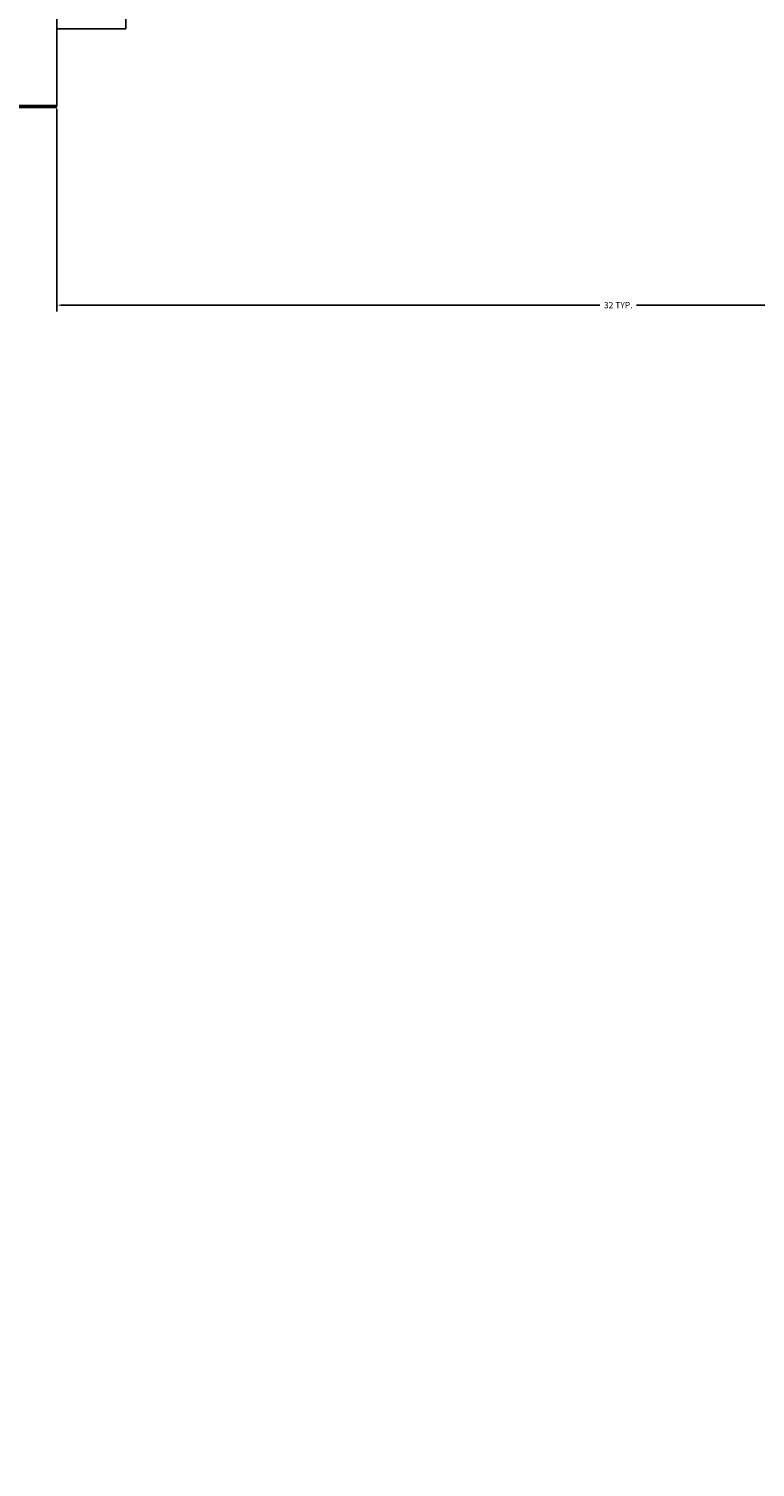
# Model space of a CAD drawing. Units: inches. Extents: x 963 to 2075, y 289 to 2657.
# Tile 92 of 98: x 1767 to 1788, y 2283 to 2325. Entities that reach past the tile are written whole.
import ezdxf

# ---------------------------------------------------------------- set-up
doc = ezdxf.new("R2010")
doc.units = ezdxf.units.IN
for name, color, linetype, lineweight in [('A-ANNO-DIMS', 2, 'Continuous', 18), ('A-DOOR', 4, 'Continuous', 25), ('A-WALL', 7, 'Continuous', 50), ('A-WALL-PATT', 8, 'Continuous', 13)]:
    doc.layers.add(name, color=color, linetype=linetype, lineweight=lineweight)
doc.styles.get("Standard").update_dxf_attribs({"font": 'arial.ttf'})
doc.dimstyles.get("Standard").update_dxf_attribs({"dimtxt": 0.18, "dimasz": 0.18, "dimexe": 0.18, "dimexo": 0.0625, "dimgap": 0.09, "dimtad": 0, "dimtih": 1, "dimtoh": 1, "dimdec": 4, "dimzin": 0, "dimdsep": 46, "dimtxsty": 'Standard', "dimcen": 0.09, "dimadec": 0, "dimazin": 0, "dimtfac": 1, "dimtdec": 4, "dimtofl": 0, "dimtmove": 0, "dimatfit": 3, "dimfxl": 1, "dimtolj": 1, "dimtzin": 0, "dimarcsym": 0})

# ---------------------------------------------------------------- blocks, each defined once
blk = doc.blocks.new('DOOR-3')
for p, q in [((2, 2.25), (2, 38.25)), ((0, 4.5), (0, 0)), ((32.386, 4.5), (32.386, 0)), ((0, 0), (0, 2.25)), ((0, 2.25), (2, 2.25)), ((32.386, 2.25), (30.386, 2.25)), ((32.386, 0), (32.386, 2.25))]:
    blk.add_line(p, q)
blk.add_arc((2, 9.059), 29.191, 346.5105, 90)
blk = doc.blocks.new('*D35')
at = {"layer": 'A-ANNO-DIMS', "color": 0, "lineweight": -2, "transparency": 16777216}
for p, q in [((1768.037, 2322.755), (1768.037, 2316.9)), ((1800.508, 2322.755), (1800.508, 2316.9)), ((1768.217, 2317.08), (1783.745, 2317.08)), ((1800.328, 2317.08), (1784.801, 2317.08))]:
    blk.add_line(p, q, dxfattribs=at)
at = {"layer": 'A-ANNO-DIMS', "color": 0, "transparency": 16777216}
for points in [[(1768.217, 2317.11), (1768.217, 2317.05), (1768.037, 2317.08)], [(1800.328, 2317.11), (1800.328, 2317.05), (1800.508, 2317.08)]]:
    blk.add_solid(points, dxfattribs=at)
at = {"layer": 'Defpoints', "color": 0, "transparency": 16777216}
for p in [(1768.037, 2322.818), (1800.508, 2322.818), (1800.508, 2317.08)]:
    blk.add_point(p, dxfattribs=at)
at = {"layer": 'A-ANNO-DIMS', "color": 0, "transparency": 16777216, "insert": (1784.273, 2317.08), "char_height": 0.18, "attachment_point": 5}
blk.add_mtext('\\A1;32 TYP.', dxfattribs=at)

msp = doc.modelspace()

# ---------------------------------------------------------------- hatches: boundary and pattern name
at = {"layer": 'A-WALL-PATT'}
h = msp.add_hatch(dxfattribs=at)
h.set_pattern_fill('ANSI32', color=256)
h.paths.add_polyline_path([(1296.922, 2558.318), (1203.922, 2558.318), (1203.922, 2493.818), (1191.533, 2493.818), (1191.533, 2489.318), (1211.063, 2489.318), (1211.063, 2492.02), (1211.063, 2493.818), (1208.422, 2493.818), (1208.422, 2553.818), (1292.422, 2553.818), (1292.422, 2538.863), (1296.922, 2538.863)])
h.paths.add_polyline_path([(1442.422, 2558.318), (1349.422, 2558.318), (1349.422, 2538.943), (1353.922, 2538.943), (1353.922, 2553.818), (1437.922, 2553.818), (1437.922, 2493.818), (1434.542, 2493.818), (1434.542, 2489.318), (1448.311, 2489.318), (1448.311, 2491.568), (1448.311, 2493.818), (1442.422, 2493.818)])
h.paths.add_polyline_path([(1415.554, 2491.568), (1415.554, 2493.818), (1340.941, 2493.818), (1340.941, 2489.318), (1371.922, 2489.318), (1371.922, 2378.318), (1367.596, 2378.318), (1367.596, 2373.818), (1371.922, 2373.818), (1371.922, 2355.185), (1376.422, 2355.185), (1376.422, 2489.318), (1415.554, 2489.318)])
h.paths.add_polyline_path([(1304.941, 2491.568), (1304.941, 2493.818), (1296.922, 2493.818), (1296.922, 2514.863), (1292.422, 2514.863), (1292.422, 2493.818), (1232.808, 2493.818), (1232.808, 2489.318), (1256.422, 2489.318), (1256.422, 2327.318), (1253.714, 2327.318), (1253.714, 2322.818), (1328.422, 2322.818), (1328.422, 2331.147), (1323.922, 2331.147), (1323.922, 2327.318), (1260.922, 2327.318), (1260.922, 2373.818), (1323.922, 2373.818), (1323.922, 2357.812), (1328.422, 2357.812), (1328.422, 2373.818), (1346.007, 2373.818), (1346.007, 2376.068), (1346.007, 2378.318), (1260.922, 2378.318), (1260.922, 2489.318), (1304.941, 2489.318)])
h.paths.add_polyline_path([(1226.654, 2327.318), (1124.422, 2327.318), (1124.422, 2347.447), (1119.922, 2347.447), (1119.922, 2322.818), (1163.422, 2322.818), (1163.422, 2305.435), (1165.672, 2305.435), (1167.922, 2305.435), (1167.922, 2322.818), (1226.654, 2322.818), (1226.654, 2325.068)])
h.paths.add_polyline_path([(1095.922, 2489.318), (1124.422, 2489.318), (1131.533, 2489.318), (1131.533, 2491.568), (1131.533, 2493.818), (1119.922, 2493.818), (1091.422, 2493.818), (1091.422, 2417.318), (1095.922, 2417.318), (1119.922, 2417.318), (1119.922, 2407.447), (1124.422, 2407.447), (1124.422, 2421.818), (1095.922, 2421.818)])
h.paths.add_polyline_path([(1512.922, 2558.318), (1508.422, 2558.318), (1508.422, 2493.818), (1503.401, 2493.818), (1503.401, 2489.318), (1508.422, 2489.318), (1508.422, 2327.318), (1376.422, 2327.318), (1376.422, 2330.273), (1371.922, 2330.273), (1371.922, 2298.744), (1376.422, 2298.744), (1376.422, 2322.818), (1508.422, 2322.818), (1508.422, 2165.318), (1504.255, 2165.318), (1504.255, 2160.818), (1508.422, 2160.818), (1508.422, 2108.318), (1512.922, 2108.318), (1512.922, 2160.818), (1516.182, 2160.818), (1516.182, 2163.068), (1516.182, 2165.318), (1512.922, 2165.318), (1512.922, 2322.818), (1644.922, 2322.818), (1644.922, 2298.744), (1649.422, 2298.744), (1649.422, 2322.818), (1649.422, 2330.944), (1647.172, 2330.944), (1644.922, 2330.944), (1644.922, 2327.318), (1512.922, 2327.318), (1512.922, 2489.318), (1516.759, 2489.318), (1516.759, 2491.568), (1516.759, 2493.818), (1512.922, 2493.818)])
h.paths.add_polyline_path([(1671.922, 2558.318), (1578.922, 2558.318), (1578.922, 2493.818), (1573.526, 2493.818), (1573.526, 2489.318), (1586.537, 2489.318), (1586.537, 2491.568), (1586.537, 2493.818), (1583.422, 2493.818), (1583.422, 2553.818), (1667.422, 2553.818), (1667.422, 2541.109), (1671.922, 2541.109)])
h.paths.add_polyline_path([(1681.257, 2493.818), (1671.922, 2493.818), (1671.922, 2517.109), (1667.422, 2517.109), (1667.422, 2493.818), (1610.218, 2493.818), (1610.218, 2489.318), (1644.922, 2489.318), (1644.922, 2357.865), (1649.422, 2357.865), (1649.422, 2373.818), (1652.203, 2373.818), (1652.203, 2375.827), (1652.203, 2378.318), (1649.422, 2378.318), (1649.422, 2489.318), (1681.257, 2489.318), (1681.257, 2491.568)])
h.paths.add_polyline_path([(1821.922, 2558.318), (1728.922, 2558.318), (1728.922, 2541), (1733.422, 2541), (1733.422, 2553.818), (1817.422, 2553.818), (1817.422, 2493.818), (1813.507, 2493.818), (1813.507, 2489.318), (1830.078, 2489.318), (1830.078, 2491.568), (1830.078, 2493.818), (1821.922, 2493.818)])
h.paths.add_polyline_path([(1794.244, 2493.818), (1717.257, 2493.818), (1717.257, 2489.318), (1760.422, 2489.318), (1760.422, 2378.318), (1674.401, 2378.318), (1674.401, 2373.818), (1692.922, 2373.818), (1692.922, 2356.954), (1697.422, 2356.954), (1697.422, 2373.818), (1760.422, 2373.818), (1760.422, 2327.318), (1697.422, 2327.318), (1697.422, 2333.341), (1692.922, 2333.341), (1692.922, 2322.818), (1768.037, 2322.818), (1768.037, 2325.068), (1768.037, 2327.318), (1764.922, 2327.318), (1764.922, 2489.318), (1794.244, 2489.318)])
h.paths.add_polyline_path([(1733.422, 2517), (1728.922, 2517), (1728.922, 2493.818), (1733.422, 2493.818)], flags=17)
h.paths.add_polyline_path([(1929.922, 2493.818), (1890.078, 2493.818), (1890.078, 2489.318), (1896.922, 2489.318), (1925.422, 2489.318), (1925.422, 2421.818), (1896.922, 2421.818), (1896.922, 2408.318), (1901.422, 2408.318), (1901.422, 2417.318), (1925.422, 2417.318), (1929.922, 2417.318)])
h.paths.add_polyline_path([(1901.422, 2348.318), (1896.922, 2348.318), (1896.922, 2327.318), (1800.423, 2327.318), (1800.423, 2322.818), (1853.422, 2322.818), (1853.422, 2309.453), (1857.922, 2309.453), (1857.922, 2322.818), (1901.422, 2322.818)])
h.paths.add_polyline_path([(1857.922, 2249.453), (1853.422, 2249.453), (1853.422, 2214.818), (1686.309, 2214.818), (1686.309, 2210.318), (1853.422, 2210.318), (1853.422, 2202.134), (1857.922, 2202.134), (1857.922, 2210.318)])
h.paths.add_polyline_path([(1857.922, 2142.134), (1853.422, 2142.134), (1853.422, 2115.422), (1841.422, 2115.422), (1841.422, 2088.531), (1841.422, 2046.949), (1845.922, 2046.949), (1845.922, 2110.922), (1905.922, 2110.922), (1905.922, 2092.517), (1910.422, 2092.517), (1910.422, 2115.422), (1857.922, 2115.422)])
h.paths.add_polyline_path([(1532.436, 1482.342), (1573.456, 1482.342), (1573.456, 1501), (1532.436, 1501)], flags=9)
h.paths.add_polyline_path([(1438.658, 1486.302), (1479.678, 1486.302), (1479.678, 1504.96), (1438.658, 1504.96)], flags=9)
h.paths.add_polyline_path([(1411.215, 1365.308), (1659.139, 1365.308), (1659.139, 1402.401), (1411.215, 1402.401)], flags=9)
h.paths.add_polyline_path([(1185.671, 2296.298), (1248.16, 2296.298), (1248.16, 2314.955), (1185.671, 2314.955)], flags=9)
h.paths.add_polyline_path([(1177.31, 2187.35), (1216.15, 2187.35), (1216.15, 2206.007), (1177.31, 2206.007)], flags=9)
h.paths.add_polyline_path([(1295.101, 1602.083), (1328.26, 1602.083), (1328.26, 1620.741), (1295.101, 1620.741)], flags=9)
h.paths.add_polyline_path([(1525.126, 2005.99), (1558.39, 2005.99), (1558.39, 2024.648), (1525.126, 2024.648)], flags=9)
h.paths.add_polyline_path([(1459.606, 1977.125), (1472.195, 1977.125), (1472.195, 1987.429), (1459.606, 1987.429)], flags=9)
h.paths.add_polyline_path([(1467.815, 2053.676), (1480.018, 2053.676), (1480.018, 2063.979), (1467.815, 2063.979)], flags=9)
h.paths.add_polyline_path([(1555.184, 2119.02), (1584.563, 2119.02), (1584.563, 2137.678), (1555.184, 2137.678)], flags=25)
h.paths.add_polyline_path([(1405.389, 2115.291), (1444.478, 2115.291), (1444.478, 2133.948), (1405.389, 2133.948)], flags=25)
h.paths.add_polyline_path([(1698.482, 2004.259), (1727.695, 2004.259), (1727.695, 2022.916), (1698.482, 2022.916)], flags=9)
h.paths.add_polyline_path([(1612.158, 1972.855), (1629.016, 1972.855), (1629.016, 1983.159), (1612.158, 1983.159)], flags=9)
h.paths.add_polyline_path([(1608.289, 2060.036), (1625.147, 2060.036), (1625.147, 2070.34), (1608.289, 2070.34)], flags=9)
h.paths.add_polyline_path([(1527.954, 1684.402), (1566.795, 1684.402), (1566.795, 1703.06), (1527.954, 1703.06)], flags=9)
h.paths.add_polyline_path([(1422.792, 1683.59), (1461.633, 1683.59), (1461.633, 1702.247), (1422.792, 1702.247)], flags=9)
h.paths.add_polyline_path([(1531.262, 1732.459), (1574.015, 1732.459), (1574.015, 1751.116), (1531.262, 1751.116)], flags=9)
h.paths.add_polyline_path([(1402.872, 1732.845), (1439.799, 1732.845), (1439.799, 1751.502), (1402.872, 1751.502)], flags=9)
h.paths.add_polyline_path([(1243.122, 1923.132), (1281.962, 1923.132), (1281.962, 1941.79), (1243.122, 1941.79)], flags=9)
h.paths.add_polyline_path([(1181.752, 1792.268), (1244.241, 1792.268), (1244.241, 1810.926), (1181.752, 1810.926)], flags=9)
h.paths.add_polyline_path([(1265.822, 1670.3), (1316.071, 1670.3), (1316.071, 1688.957), (1265.822, 1688.957)], flags=9)
h.paths.add_polyline_path([(1140.263, 1676.054), (1179.104, 1676.054), (1179.104, 1694.711), (1140.263, 1694.711)], flags=9)
h.paths.add_polyline_path([(1107.49, 1490.889), (1143.374, 1490.889), (1143.374, 1509.546), (1107.49, 1509.546)], flags=9)
h.paths.add_polyline_path([(1217.584, 1483.899), (1246.741, 1483.899), (1246.741, 1502.556), (1217.584, 1502.556)], flags=9)
h.paths.add_polyline_path([(1389.21, 1486.919), (1418.367, 1486.919), (1418.367, 1505.576), (1389.21, 1505.576)], flags=9)
h.paths.add_polyline_path([(1672.208, 1602.083), (1705.366, 1602.083), (1705.366, 1620.741), (1672.208, 1620.741)], flags=9)
h.paths.add_polyline_path([(1752.082, 1522.638), (1781.24, 1522.638), (1781.24, 1541.295), (1752.082, 1541.295)], flags=9)
h.paths.add_polyline_path([(1848.275, 1491.26), (1884.158, 1491.26), (1884.158, 1509.918), (1848.275, 1509.918)], flags=9)
h.paths.add_polyline_path([(1822.47, 1685.62), (1861.31, 1685.62), (1861.31, 1704.278), (1822.47, 1704.278)], flags=9)
h.paths.add_polyline_path([(1713.195, 1672.232), (1763.444, 1672.232), (1763.444, 1690.889), (1713.195, 1690.889)], flags=9)
h.paths.add_polyline_path([(1736.619, 1790.578), (1799.109, 1790.578), (1799.109, 1809.235), (1736.619, 1809.235)], flags=9)
h.paths.add_polyline_path([(1691.491, 1916.355), (1730.332, 1916.355), (1730.332, 1935.013), (1691.491, 1935.013)], flags=9)
h.paths.add_polyline_path([(1764.872, 1973.922), (1794.306, 1973.922), (1794.306, 1992.58), (1764.872, 1992.58)], flags=9)
h.paths.add_polyline_path([(1767.854, 2034.017), (1797.288, 2034.017), (1797.288, 2052.674), (1767.854, 2052.674)], flags=9)
h.paths.add_polyline_path([(1851.593, 2060.331), (1880.751, 2060.331), (1880.751, 2078.989), (1851.593, 2078.989)], flags=25)
h.paths.add_polyline_path([(1688.491, 2086.874), (1727.332, 2086.874), (1727.332, 2105.531), (1688.491, 2105.531)], flags=9)
h.paths.add_polyline_path([(1537.743, 2293.581), (1580.495, 2293.581), (1580.495, 2312.239), (1537.743, 2312.239)], flags=25)
h.paths.add_polyline_path([(1425.587, 2296.109), (1468.34, 2296.109), (1468.34, 2314.766), (1425.587, 2314.766)], flags=25)
h.paths.add_polyline_path([(1278.518, 2004.184), (1307.72, 2004.184), (1307.72, 2022.841), (1278.518, 2022.841)], flags=9)
h.paths.add_polyline_path([(1193.282, 1973.635), (1222.715, 1973.635), (1222.715, 1992.292), (1193.282, 1992.292)], flags=9)
h.paths.add_polyline_path([(1192.411, 2040.577), (1221.845, 2040.577), (1221.845, 2059.234), (1192.411, 2059.234)], flags=9)
h.paths.add_polyline_path([(1130.603, 1951.393), (1159.76, 1951.393), (1159.76, 1970.05), (1130.603, 1970.05)], flags=9)
h.paths.add_polyline_path([(1132.827, 2052.494), (1161.984, 2052.494), (1161.984, 2071.151), (1132.827, 2071.151)], flags=9)
h.paths.add_polyline_path([(1265.128, 2334.619), (1315.377, 2334.619), (1315.377, 2353.277), (1265.128, 2353.277)], flags=25)
h.paths.add_polyline_path([(1136.741, 2330.785), (1175.582, 2330.785), (1175.582, 2349.443), (1136.741, 2349.443)], flags=9)
h.paths.add_polyline_path([(1287.422, 2417.204), (1320.58, 2417.204), (1320.58, 2435.861), (1287.422, 2435.861)], flags=25)
h.paths.add_polyline_path([(1430.988, 2329.159), (1469.828, 2329.159), (1469.828, 2347.816), (1430.988, 2347.816)], flags=25)
h.paths.add_polyline_path([(1525.424, 2329.213), (1564.264, 2329.213), (1564.264, 2347.87), (1525.424, 2347.87)], flags=25)
h.paths.add_polyline_path([(1684.525, 2382.799), (1717.683, 2382.799), (1717.683, 2401.457), (1684.525, 2401.457)], flags=25)
h.paths.add_polyline_path([(1704.805, 2340.293), (1755.054, 2340.293), (1755.054, 2358.95), (1704.805, 2358.95)], flags=25)
h.paths.add_polyline_path([(1694.113, 2287.757), (1756.602, 2287.757), (1756.602, 2306.414), (1694.113, 2306.414)], flags=9)
h.paths.add_polyline_path([(1815.778, 2329.861), (1854.618, 2329.861), (1854.618, 2348.518), (1815.778, 2348.518)], flags=9)
h.paths.add_polyline_path([(1842.873, 2514.256), (1878.756, 2514.256), (1878.756, 2532.914), (1842.873, 2532.914)], flags=9)
h.paths.add_polyline_path([(1769.513, 2531.447), (1798.671, 2531.447), (1798.671, 2550.104), (1769.513, 2550.104)], flags=25)
h.paths.add_polyline_path([(1594.772, 2518.468), (1623.93, 2518.468), (1623.93, 2537.125), (1594.772, 2537.125)], flags=25)
h.paths.add_polyline_path([(1520.723, 2516.185), (1556.606, 2516.185), (1556.606, 2534.842), (1520.723, 2534.842)], flags=25)
h.paths.add_polyline_path([(1464.456, 2516.694), (1500.34, 2516.694), (1500.34, 2535.351), (1464.456, 2535.351)], flags=25)
h.paths.add_polyline_path([(1365.696, 2528.97), (1394.854, 2528.97), (1394.854, 2547.627), (1365.696, 2547.627)], flags=25)
h.paths.add_polyline_path([(1222.838, 2516.231), (1251.995, 2516.231), (1251.995, 2534.889), (1222.838, 2534.889)], flags=25)
h.paths.add_polyline_path([(1104.545, 2509.6), (1140.429, 2509.6), (1140.429, 2528.257), (1104.545, 2528.257)], flags=9)

# ---------------------------------------------------------------- linework, layer by layer
at = {"layer": 'A-WALL'}
msp.add_line((1692.922, 2322.818), (1768.037, 2322.818), dxfattribs=at)

# ---------------------------------------------------------------- block references
at = {"layer": 'A-DOOR'}
msp.add_blockref('DOOR-3', (1768.037, 2322.818), dxfattribs=at)

# ---------------------------------------------------------------- dimensions: what is measured, and where the dimension line sits
at = {"layer": 'A-ANNO-DIMS'}
dim = msp.add_linear_dim(base=(1800.508, 2317.08), p1=(1768.037, 2322.818), p2=(1800.508, 2322.818), text='<> TYP.', dimstyle='Standard', override={"dimdec": 0, "dimlfac": 1, "dimrnd": 0, "dimzin": 0, "dimdsep": 46, "dimlunit": 2}, dxfattribs=at)
dim.commit()
dim.dimension.update_dxf_attribs({"geometry": '*D35', "text_midpoint": (1784.273, 2317.08)})

doc.saveas('drawing.dxf')
